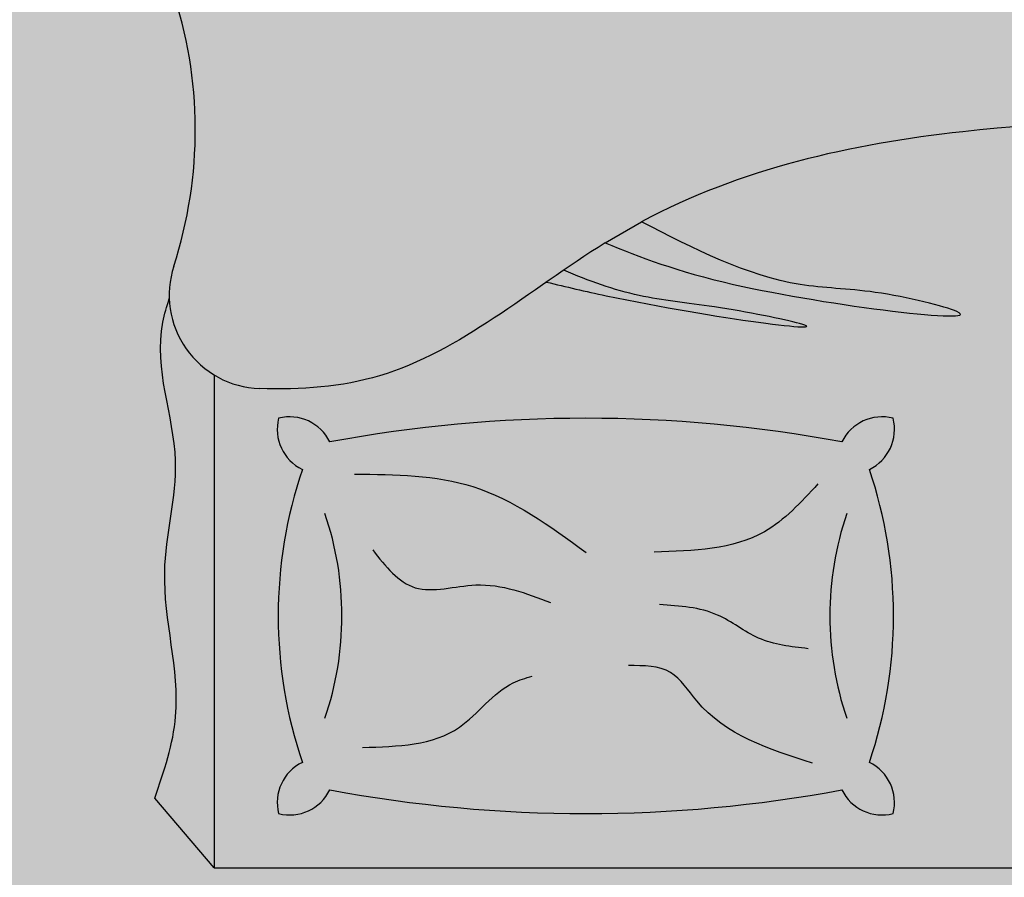
# Model space of a CAD drawing. Units: inches. Extents: x 1704 to 6393, y -157 to 1172.
# Tile 34 of 122: x 2488 to 2529, y 112 to 148. Entities that reach past the tile are written whole.
import ezdxf

# ---------------------------------------------------------------- set-up
doc = ezdxf.new("R2010")
doc.units = ezdxf.units.IN
doc.header["$MEASUREMENT"] = 0
for name, color, linetype, lineweight in [('A-ANNO-DIMS', 7, 'Continuous', 13), ('A-FURN', 8, 'Continuous', 18), ('estofado', 7, 'Continuous', 25)]:
    doc.layers.add(name, color=color, linetype=linetype, lineweight=lineweight)
doc.layers.add('A-FLOR-PATT', color=7, linetype='Continuous', lineweight=13, true_color=0xf2f2f2)
doc.styles.get("Standard").update_dxf_attribs({"font": 'arial.ttf'})
doc.dimstyles.get("Standard").update_dxf_attribs({"dimtxt": 6, "dimasz": 2, "dimexe": 0.18, "dimexo": 0.0625, "dimgap": 0.09, "dimtad": 0, "dimtih": 1, "dimtoh": 1, "dimdec": 1, "dimzin": 0, "dimdsep": 46, "dimlunit": 3, "dimtxsty": 'Standard', "dimblk": 'ARCHTICK', "dimcen": 0.09, "dimadec": 0, "dimazin": 0, "dimtfac": 1, "dimtdec": 1, "dimtofl": 0, "dimtmove": 0, "dimatfit": 3, "dimfxl": 1, "dimtolj": 1, "dimtzin": 0, "dimarcsym": 0})

# ---------------------------------------------------------------- blocks, each defined once
blk = doc.blocks.new('Cama Box Regencia LOLA')
at = {"layer": 'estofado', "ltscale": 0.2}
h = blk.add_hatch(color=256, dxfattribs=at)
h.dxf.hatch_style = 1
h.set_gradient(color1=(240, 232, 219), color2=(213, 190, 154), one_color=1, tint=0.7200000286102295, name='CURVED')
edge = h.paths.add_edge_path()
edge.add_spline(control_points=[(0.343533776195045, -0.8455058148597345), (0.2879313990920309, -0.8167160606696484), (0.2054770794474052, -0.7744470032542381), (0.0954193394759386, -0.7742416952675626), (-0.0885363502328574, -0.7276964167006668), (0.2428192566063672, -0.7672518992321216), (0.345087521536243, -0.8076697826234067), (0.3825206986321063, -0.8228555492498799)], knot_values=[0.0056315103357428, 0.0056315103357428, 0.0056315103357428, 0.0056315103357428, 0.1860138916206105, 0.2660015162584448, 0.3570871810327863, 0.5963901805690979, 0.739731738908988, 0.739731738908988, 0.739731738908988, 0.739731738908988], degree=3, periodic=0)
edge.add_spline(control_points=[(0.3825206986325611, -0.8228555492497662), (0.3974221570828149, -0.8135511441712424), (0.4121061736600496, -0.8037181558521524), (0.4266849906532571, -0.7937075488799225)], knot_values=[1.358237767273279, 1.358237767273279, 1.358237767273279, 1.358237767273279, 1.409915662372559, 1.409915662372559, 1.409915662372559, 1.409915662372559], degree=3, periodic=0)
edge.add_spline(control_points=[(0.4266849905698109, -0.7937075489369932), (0.3998777739682282, -0.7821381809783361), (0.3476761897024971, -0.7634757898491671), (0.2670618099601825, -0.7565375622627358), (0.0835725072796549, -0.7192994417154637), (0.288524529784695, -0.7446405493717521), (0.4247448861246994, -0.7759943071475277), (0.4449816270193879, -0.7810438091316882)], knot_values=[0.1043639306803623, 0.1043639306803623, 0.1043639306803623, 0.1043639306803623, 0.1896363068641149, 0.2696239315019491, 0.3607095962762907, 0.6000125958126024, 0.6446217338078729, 0.6446217338078729, 0.6446217338078729, 0.6446217338078729], degree=3, periodic=0)
edge.add_spline(control_points=[(0.4449816270197289, -0.7810438091316882), (0.5029779388527232, -0.7406836481117695), (0.5966687145296419, -0.6736247633211292), (0.7071737530245628, -0.6656573253703187), (0.7517012483331201, -0.6672238302253392)], knot_values=[1.43159032281798, 1.43159032281798, 1.43159032281798, 1.43159032281798, 1.63814180148235, 1.770695287284994, 1.770695287284994, 1.770695287284994, 1.770695287284994], degree=3, periodic=0)
edge.add_arc((0.7481853615017826, -0.767162003811734), 0.0999999999999888, 58.7920033978138, 87.98512997550938, ccw=False)
edge.add_line((0.8000000000000682, -0.6816328085782289), (0.8000000000000682, -0.154802362840428))
edge.add_line((0.8000000000000682, -0.154802362840428), (-0.7999999999999546, -0.154802362840428))
edge.add_line((-0.7999999999999546, -0.154802362840428), (-0.8000000000000682, -0.7409839258539819))
edge.add_spline(control_points=[(-0.799999999999841, -0.7409839258539251), (-0.7846451382113174, -0.74846387981205), (-0.7568940913494089, -0.7651582159765554), (-0.7559936909002545, -0.8096905380045313), (-0.7049413305308008, -0.8142555457367848), (-0.7013836936888538, -0.8139988647640733)], knot_values=[0.0122267587020837, 0.0122267587020837, 0.0122267587020837, 0.0122267587020837, 0.0594720782072034, 0.1062176618094138, 0.134458043575382, 0.134458043575382, 0.134458043575382, 0.134458043575382], degree=3, periodic=0)
edge.add_spline(control_points=[(-0.7013836936890812, -0.8139988647637892), (-0.6428309483887916, -0.8132695376718857), (-0.532520673001045, -0.8118955240036598), (-0.2390712668254764, -0.6717984706609172), (-0.3892411364554391, -0.7557901092520752), (-0.4591093260188473, -0.8070101468627512), (-0.5571511178645779, -0.795652750469742), (-0.608497950975675, -0.8409486634728295), (-0.6632498050151981, -0.8266781836207997), (-0.6991149398675134, -0.8254126024436914), (-0.719552182989446, -0.8246914287938125)], knot_values=[0, 0, 0, 0, 0.2187005959148062, 0.4120203559900679, 0.4786136596093368, 0.6046444033330721, 0.6969970394608519, 0.7456449795902803, 0.7925683322559657, 0.8547274388453192, 0.8547274388453192, 0.8547274388453192, 0.8547274388453192], degree=3, periodic=0)
edge.add_spline(control_points=[(-0.7195521829781911, -0.824691428792164), (-0.7293124663336812, -0.8248308281530967), (-0.7545977292818407, -0.8216412233076653), (-0.7742556984202338, -0.794819860189591), (-0.7939222919129634, -0.7820064600295497), (-0.799999999999841, -0.7800193173443404)], knot_values=[0.1564883932805935, 0.1564883932805935, 0.1564883932805935, 0.1564883932805935, 0.184397548386913, 0.2313764834161266, 0.2505984550882281, 0.2505984550882281, 0.2505984550882281, 0.2505984550882281], degree=3, periodic=0)
edge.add_line((-0.8000000000000682, -0.7800193173444541), (-0.7999999999999546, -0.8218505664627286))
edge.add_spline(control_points=[(-0.7999999999999546, -0.8218505664625013), (-0.7938082505512511, -0.8290217081292894), (-0.7673857405620766, -0.8512914803976059), (-0.7619109683460011, -0.8661369353891359), (-0.6555700939965164, -0.8510070218793543), (-0.7139793977868294, -0.8637526923380391), (-0.7379026254519659, -0.8623504601624176), (-0.7688129786438367, -0.8813042143888196), (-0.7854260296310259, -0.8561610219318254), (-0.7961930533253962, -0.8566031243811949), (-0.7999999999999546, -0.8573491405791173)], knot_values=[0.0595743221876141, 0.0595743221876141, 0.0595743221876141, 0.0595743221876141, 0.08075289116965, 0.1037414994169835, 0.1697200936249022, 0.1760361327243865, 0.2071371586311508, 0.2404744334261798, 0.2623408547027293, 0.2736604507987723, 0.2736604507987723, 0.2736604507987723, 0.2736604507987723], degree=3, periodic=0)
edge.add_line((-0.7999999999999546, -0.8573491405791173), (-0.8000000000000682, -0.9113562424721521))
edge.add_spline(control_points=[(-0.8000000000000682, -0.9113562424720385), (-0.7937204054647964, -0.9077594990848183), (-0.7710343135782978, -0.8978798065321029), (-0.7213062468074442, -0.9144666877443228), (-0.6268586829058905, -0.862430497409548), (-0.6896594748232019, -0.9045634991654196), (-0.7483442493064559, -0.9189273406958591), (-0.7835301183422417, -0.922920432793262), (-0.7896301351460125, -0.9477657000142585), (-0.7975786973822779, -0.955260590410262), (-0.8000000000001818, -0.9571831923294098)], knot_values=[0.0138560263374175, 0.0138560263374175, 0.0138560263374175, 0.0138560263374175, 0.0348737775836104, 0.0888666909546002, 0.1078792274429341, 0.1267378491223226, 0.1587140219647659, 0.1937574699451985, 0.2174867851300671, 0.2267221218327879, 0.2267221218327879, 0.2267221218327879, 0.2267221218327879], degree=3, periodic=0)
edge.add_line((-0.7999999999999546, -0.957183192329296), (-0.7999999999999546, -1.145824641594742))
edge.add_spline(control_points=[(-0.8000000000002955, -1.145824641594913), (-0.7271039467997298, -1.094596787649038), (-0.4885706936571524, -0.9465888221489535), (-0.0701640902225336, -0.9707493165000187), (0.237911901821235, -0.902164522332157), (0.3435337762145991, -0.845505814843193)], knot_values=[0.1168958193629841, 0.1168958193629841, 0.1168958193629841, 0.1168958193629841, 0.3797203297758731, 0.9577018633805092, 1.31379338443587, 1.31379338443587, 1.31379338443587, 1.31379338443587], degree=3, periodic=0)
h.paths.add_polyline_path([(-0.6766340706021765, -0.6101327540145576, -0.3575266660906883), (-0.7312746368313583, -0.6354535276154252, -0.3575266660894137), (-0.7059538632299791, -0.5808129613865844, -0.1647847126465284), (-0.7059538632300928, -0.2676124402649407, -0.3575266660890756), (-0.7312746368312446, -0.2129718740360431, -0.3575266660908716), (-0.6766340706020629, -0.2382926476369676, -0.0925607043966334), (-0.1295169377724505, -0.2382926476369107, -0.3575266660898965), (-0.0748763715433825, -0.2129718740360431, -0.3575266660894428), (-0.1001971451446479, -0.2676124402649407, -0.1647847126465285), (-0.1001971451445343, -0.5808129613865844, -0.3575266660890756), (-0.0748763715433825, -0.6354535276154821, -0.3575266660898962), (-0.1295169377724505, -0.6101327540146145, -0.0925607043966531)], flags=16)
h.paths.add_polyline_path([(0.0748763715433825, -0.6354535276157094, -0.3575266660910266), (0.1001971451446479, -0.5808129613865844, -0.1647847126465284), (0.1001971451445343, -0.2676124402649407, -0.3575266660890757), (0.0748763715433825, -0.2129718740360431, -0.3575266660898962), (0.1295169377724505, -0.2382926476369107, -0.0925607043966334), (0.6766340706020629, -0.2382926476369676, -0.3575266660908718), (0.7312746368312446, -0.2129718740360431, -0.3575266660894425), (0.7059538632299791, -0.2676124402649407, -0.1647847126465283), (0.7059538632300928, -0.5808129613865844, -0.3575266660890756), (0.7312746368312446, -0.6354535276154821, -0.3575266660908716), (0.6766340706020629, -0.6101327540145576, -0.0925607043966335), (0.1295169377724505, -0.6101327540146145, -0.3575266660906303)], flags=16)
h = blk.add_hatch(color=256, dxfattribs=at)
h.dxf.hatch_style = 1
h.set_gradient(color1=(240, 232, 219), color2=(213, 190, 154), one_color=1, tint=0.7200000286102295)
edge = h.paths.add_edge_path()
edge.add_spline(control_points=[(0.8481164014890509, -0.7634488855285327), (0.8506728373771466, -0.7550468983013161), (0.868679602201837, -0.6953776187201015), (0.8253488717913342, -0.6001498518888299), (0.8674912876568897, -0.4595932758330151), (0.8269013755603964, -0.3369378214810581), (0.8537222782124445, -0.258285373872468), (0.8635971996978923, -0.2293271111754507)], knot_values=[0, 0, 0, 0, 0.0246217641678395, 0.1732110090087366, 0.2929197011275091, 0.4476746021509216, 0.5378548332073604, 0.5378548332073604, 0.5378548332073604, 0.5378548332073604], degree=3, periodic=0)
edge.add_line((0.8635971996978923, -0.229327111175337), (0.8000000000001818, -0.1548023628403712))
edge.add_line((0.8000000000001818, -0.1548023628403712), (0.8000000000000682, -0.681632808574193))
edge.add_arc((0.7481853615026921, -0.7671620038083234), 0.0999999999999888, 2.1279492292164264, 58.79200339844499, ccw=False)
h = blk.add_hatch(color=256, dxfattribs=at)
h.dxf.hatch_style = 1
h.set_gradient(color1=(106, 82, 42), color2=(160, 123, 64), one_color=1, tint=0.4399999976158142, name='CURVED')
h.paths.add_polyline_path([(0.7059538632300928, -0.2676124402650544, 0.3575266660910843), (0.731274636831131, -0.2129718740358157, 0.3575266660898384), (0.6766340706021765, -0.2382926476369107, 0.092560704396653), (0.1295169377724505, -0.2382926476369676, 0.3575266660900799), (0.0748763715433825, -0.2129718740360431, 0.3575266660883129), (0.1001971451444206, -0.2676124402648838, 0.1647847126464969), (0.1001971451445343, -0.5808129613864708, 0.3575266660914516), (0.0748763715433825, -0.6354535276157094, 0.3575266660906303), (0.1295169377724505, -0.6101327540146145, 0.0925607043966335), (0.6766340706020629, -0.6101327540146145, 0.3575266660906881), (0.7312746368312446, -0.6354535276154821, 0.3575266660886796), (0.7059538632300928, -0.5808129613866413, 0.1647847126464968)])
h = blk.add_hatch(color=256, dxfattribs=at)
h.dxf.hatch_style = 1
h.set_gradient(color1=(206, 178, 131), color2=(227, 212, 186), one_color=1, tint=0.8100000023841857, name='CYLINDER')
edge = h.paths.add_edge_path()
edge.add_arc((0.7481853614966667, -0.7671620038115634), 0.0999999999999888, 342.0511336145294, 447.9851299725766)
edge.add_spline(control_points=[(0.7517012483331201, -0.6672238302253392), (0.7071737530245628, -0.6656573253703187), (0.5966687145298692, -0.6736247633211292), (0.5029779388527232, -0.7406836481117125), (0.4449816270195015, -0.7810438091316314)], knot_values=[1.431590322817835, 1.431590322817835, 1.431590322817835, 1.431590322817835, 1.564143808620479, 1.770695287284994, 1.770695287284994, 1.770695287284994, 1.770695287284994], degree=3, periodic=0)
edge.add_spline(control_points=[(0.4449816270195015, -0.7810438091316314), (0.4388957332065502, -0.7852790380018178), (0.4327996148541616, -0.7895089160493285), (0.4266849906533708, -0.7937075488798087)], knot_values=[1.409915662372814, 1.409915662372814, 1.409915662372814, 1.409915662372814, 1.431590322817835, 1.431590322817835, 1.431590322817835, 1.431590322817835], degree=3, periodic=0)
edge.add_spline(control_points=[(0.4266849906533708, -0.7937075488798087), (0.4121061736600496, -0.8037181558521524), (0.3974221570825875, -0.8135511441712991), (0.38252069863222, -0.8228555492498799)], knot_values=[1.358237767273037, 1.358237767273037, 1.358237767273037, 1.358237767273037, 1.409915662372815, 1.409915662372815, 1.409915662372815, 1.409915662372815], degree=3, periodic=0)
edge.add_line((0.3825206986330158, -0.8228555492493114), (0.343533776286904, -0.8455058148063584))
edge.add_spline(control_points=[(0.3435337761924302, -0.8455058148550165), (0.2379119018048641, -0.902164522335795), (-0.0701640902311738, -0.9707493164995071), (-0.4885706936571524, -0.9465888221488967), (-0.7271039467997298, -1.094596787649038), (-0.8000000000000682, -1.145824641594742)], knot_values=[0.1168958193630798, 0.1168958193630798, 0.1168958193630798, 0.1168958193630798, 0.472987340393773, 1.050968873998409, 1.313793384411202, 1.313793384411202, 1.313793384411202, 1.313793384411202], degree=3, periodic=0)
edge.add_spline(control_points=[(-0.8000000000000682, -1.145824641594742), (-0.8038896190357718, -1.14855807951244), (-0.8077744942224853, -1.151305646504738), (-0.8116551946761774, -1.154065647517199)], knot_values=[0.1028719158199011, 0.1028719158199011, 0.1028719158199011, 0.1028719158199011, 0.1168958193630799, 0.1168958193630799, 0.1168958193630799, 0.1168958193630799], degree=3, periodic=0)
edge.add_arc((-0.7536973518524519, -1.235557294053705), 0.1000000000000352, 125.4208969883762, 169.6981795679068)
edge.add_spline(control_points=[(-0.852085287466366, -1.217673946333093), (-0.8521399740518518, -1.217974812833915), (-0.8565649010855622, -1.242328483616745), (-0.8662697220019026, -1.297321141147904), (-0.8487158298532904, -1.34896742172242), (-0.8348745804664758, -1.381844109035796)], knot_values=[0.3128349436863077, 0.3128349436863077, 0.3128349436863077, 0.3128349436863077, 0.3137509534211996, 0.386958004641742, 0.4759027329026081, 0.4759027329026081, 0.4759027329026081, 0.4759027329026081], degree=3, periodic=0)
edge.add_spline(control_points=[(-0.8348745804664758, -1.38184410903591), (-0.8226532004149476, -1.367823298399059), (-0.8056354908857201, -1.352141651537124), (-0.7460155199962628, -1.32170802000337)], knot_values=[0.0062456970656236, 0.0062456970656236, 0.0062456970656236, 0.0062456970656236, 0.0554759259147193, 0.0554759259147193, 0.0554759259147193, 0.0554759259147193], degree=3, periodic=0)
edge.add_spline(control_points=[(-0.7460155200169539, -1.321708019985464), (-0.6188339616464873, -1.25080943574278), (-0.3488365122128698, -1.179158668568902), (0.0338148848931041, -1.279726484458706), (0.3977250465933366, -1.412092721352792), (0.6449024721503065, -1.106270719748692), (0.7873766543807506, -1.256744909425322), (0.8547271521993025, -1.327877176513538)], knot_values=[0.0991852523588446, 0.0991852523588446, 0.0991852523588446, 0.0991852523588446, 0.5236467270390676, 0.9270872950244264, 1.289918234564769, 1.564439021262726, 1.810554634340498, 1.810554634340498, 1.810554634340498, 1.810554634340498], degree=3, periodic=0)
edge.add_arc((0.5509678495186563, -1.223443291813453), 0.3212104454069235, 341.0267878798241, 383.7782184284114)
edge.add_arc((1.292676354991499, -0.9435407756057543), 0.4723459732861395, 162.0511336103901, 198.5657216587827, ccw=False)
h = blk.add_hatch(color=256, dxfattribs=at)
h.dxf.hatch_style = 1
h.set_gradient(color1=(240, 232, 219), color2=(137, 106, 57), one_color=1, tint=0.3799999952316284, name='CURVED')
edge = h.paths.add_edge_path()
edge.add_spline(control_points=[(0.4449816270193879, -0.7810438091316882), (0.4247448861246994, -0.7759943071475277), (0.288524529784695, -0.7446405493717521), (0.0835725072796549, -0.7192994417154637), (0.2670618099601825, -0.7565375622627358), (0.3476761897024971, -0.7634757898491671), (0.3998777739682282, -0.7821381809783361), (0.4266849905698109, -0.7937075489369932)], knot_values=[0.1043639306803623, 0.1043639306803623, 0.1043639306803623, 0.1043639306803623, 0.1489730686756328, 0.3882760682119444, 0.479361732986286, 0.5593493576241202, 0.6446217338078729, 0.6446217338078729, 0.6446217338078729, 0.6446217338078729], degree=3, periodic=0)
edge.add_spline(control_points=[(0.4266849906528023, -0.7937075488800929), (0.4327996148537068, -0.7895089160495559), (0.4388957332062092, -0.7852790380020452), (0.4449816270192742, -0.781043809131802)], knot_values=[1.409915662372559, 1.409915662372559, 1.409915662372559, 1.409915662372559, 1.43159032281798, 1.43159032281798, 1.43159032281798, 1.43159032281798], degree=3, periodic=0)
h = blk.add_hatch(color=256, dxfattribs=at)
h.dxf.hatch_style = 1
h.set_gradient(color1=(240, 232, 219), color2=(137, 106, 57), one_color=1, tint=0.3799999952316284, name='CURVED')
edge = h.paths.add_edge_path()
edge.add_spline(control_points=[(0.3825206986321063, -0.8228555492498799), (0.345087521536243, -0.8076697826234067), (0.2428192566063672, -0.7672518992321216), (-0.0885363502328574, -0.7276964167006668), (0.0954193394759386, -0.7742416952675626), (0.2054770794474052, -0.7744470032542381), (0.2879313990920309, -0.8167160606696484), (0.343533776195045, -0.8455058148597345)], knot_values=[0.0056315103357428, 0.0056315103357428, 0.0056315103357428, 0.0056315103357428, 0.1489730686756328, 0.3882760682119444, 0.479361732986286, 0.5593493576241202, 0.739731738908988, 0.739731738908988, 0.739731738908988, 0.739731738908988], degree=3, periodic=0)
edge.add_line((0.343533776195045, -0.8455058148597913), (0.3825206986321063, -0.8228555492498799))
for p, q in [((0.8000000000000682, -0.154802362840428), (0.8635971996978923, -0.2293271111754507)), ((0.3825206986321063, -0.8228555492498799), (0.343533776195045, -0.8455058148597913))]:
    blk.add_line(p, q, dxfattribs=at)
blk.add_lwpolyline([(0.8000000000000682, -0.6816328085741361), (0.8000000000000682, -0.154802362840428), (-0.7999999999999546, -0.154802362840428), (-0.7999999999999546, -0.7409839258540956)], dxfattribs=at)
for centre, radius, start, end in [((0.120860229745972, -0.2248498560688859), 0.047493175008304, 165.516646303857, 244.209945069049), ((0.0867543535765663, -0.2589557322385758), 0.047493175008304, 25.79005493108792, 104.4833536962803), ((0.4030755041873136, -1.703357436968531), 1.490385562932656, 79.42346065608726, 100.5765393439197), ((0.7193966547980608, -0.2589557322385758), 0.047493175008304, 75.51664630371964, 154.2099450689121), ((0.6852907786285414, -0.2248498560688859), 0.047493175008304, 295.790054930951, 14.48335369614292), ((0.562460708312642, -0.4242127008258194), 0.4880688921049917, 161.2852469077218, 198.7147530922607), ((0.243690300061985, -0.4242127008258194), 0.4880688921049917, 341.2852469077393, 18.71475309227822), ((-0.19631084963396, -0.4242127008257626), 0.3387897965243698, 341.1598423418016, 18.84015765820971), ((1.002461858008359, -0.4242127008257626), 0.3387897965243698, 161.1598423417902, 198.8401576581983), ((0.120860229745972, -0.6235755455826393), 0.047493175008304, 115.790054930951, 194.4833536961429), ((0.6852907786285414, -0.6235755455826393), 0.047493175008304, 345.516646303857, 64.20994506904903), ((0.0867543535765663, -0.5894696694129494), 0.047493175008304, 255.5166463037197, 334.2099450689121), ((0.4030755041873136, 0.8549320353169491), 1.490385562932656, 259.4234606560803, 280.5765393439127), ((0.7193966547980608, -0.5894696694129494), 0.047493175008304, 205.7900549310879, 284.4833536962804), ((0.7481853615029195, -0.7671620038083234), 0.1, 342.0511336116027, 87.98512997616182), ((1.292676354991613, -0.9435407756055268), 0.4723459732861117, 162.0511336104213, 198.5657216589983)]:
    blk.add_arc(centre, radius, start, end, dxfattribs=at)
for points, knots in [([(0.8635971996978923, -0.2293271111754507), (0.8537222782124445, -0.258285373872468), (0.8269013755603964, -0.3369378214810581), (0.8674912876568897, -0.4595932758330151), (0.8253488717913342, -0.6001498518888299), (0.868679602201837, -0.6953776187201015), (0.8506728373771466, -0.7550468983013161), (0.8481164014890509, -0.7634488855285327)], [0, 0, 0, 0, 0.0901802310564388, 0.2449351320798513, 0.3646438241986237, 0.5132330690395209, 0.5378548332073604, 0.5378548332073604, 0.5378548332073604, 0.5378548332073604]), ([(0.1609929429250769, -0.2668120520876869), (0.207361296664481, -0.2816189425177519), (0.2673465842344797, -0.3007741531050562), (0.3100088172549912, -0.3711986237053177), (0.3410959220547441, -0.371113456673647), (0.3573768361287648, -0.371068853062809)], [0, 0, 0, 0, 0.1404794637529129, 0.1817338842404631, 0.2270973195475621, 0.2270973195475621, 0.2270973195475621, 0.2270973195475621]), ([(0.641547568925148, -0.2836087781224137), (0.6039704843628328, -0.2846768301159754), (0.539944686002343, -0.2864966328594507), (0.4983244357833337, -0.3487001107148991), (0.4673537235191868, -0.3577134183149331), (0.460449429265168, -0.3597227530484019)], [0, 0, 0, 0, 0.1057518620258909, 0.1801855432155129, 0.2015394496060149, 0.2015394496060149, 0.2015394496060149, 0.2015394496060149]), ([(0.1657269282603693, -0.3891622340328808), (0.1839821155447316, -0.3912290170364152), (0.2191851220416109, -0.3952145677934529), (0.2641538569791404, -0.4324302667024541), (0.3028411853428648, -0.4348886966416372), (0.3243911361614664, -0.4362581125853354)], [0, 0, 0, 0, 0.0540396012867365, 0.1042090889319622, 0.1672963371706364, 0.1672963371706364, 0.1672963371706364, 0.1672963371706364]), ([(0.630774277431101, -0.4946666993113809), (0.6169895699779718, -0.4772535648042688), (0.5885015945383536, -0.441266950663047), (0.5131074616321869, -0.4662255111125919), (0.4667910825139399, -0.4484404284426592), (0.4408934738504513, -0.4384959742387196)], [0, 0, 0, 0, 0.0606588350328579, 0.1253597443752535, 0.2074214353097695, 0.2074214353097695, 0.2074214353097695, 0.2074214353097695]), ([(0.1552772464440295, -0.5652394970176715), (0.1730924483668451, -0.5457941389807961), (0.2188221854511549, -0.4958799637506091), (0.2880058022633399, -0.4937226941133118), (0.3302371516485891, -0.4924058446629829)], [0, 0, 0, 0, 0.0765478869158952, 0.1964903209174588, 0.1964903209174588, 0.1964903209174588, 0.1964903209174588]), ([(0.6501439432536245, -0.5758072434303472), (0.6067249420939599, -0.5753127958675333), (0.5155219215609228, -0.5742741927209986), (0.4416129136043037, -0.5203678897559305), (0.402889750189047, -0.4921247481343585)], [0, 0, 0, 0, 0.1270530108164939, 0.2668789710677518, 0.2668789710677518, 0.2668789710677518, 0.2668789710677518]), ([(0.38252069863222, -0.8228555492498799), (0.4632317710900225, -0.7724599107979202), (0.5727651217678158, -0.6753482176968646), (0.7071737530245628, -0.6656573253703187), (0.7517012483331201, -0.6672238302253392)], [1.358237767273037, 1.358237767273037, 1.358237767273037, 1.358237767273037, 1.63814180148235, 1.770695287284994, 1.770695287284994, 1.770695287284994, 1.770695287284994]), ([(0.4449816270193879, -0.7810438091316882), (0.4247448861246994, -0.7759943071475277), (0.288524529784695, -0.7446405493717521), (0.0835725072796549, -0.7192994417154637), (0.2670618099601825, -0.7565375622627358), (0.3476761897024971, -0.7634757898491671), (0.3998777739682282, -0.7821381809783361), (0.4266849905698109, -0.7937075489369932)], [0.1043639306803623, 0.1043639306803623, 0.1043639306803623, 0.1043639306803623, 0.1489730686756328, 0.3882760682119444, 0.479361732986286, 0.5593493576241202, 0.6446217338078729, 0.6446217338078729, 0.6446217338078729, 0.6446217338078729]), ([(0.3825206986321063, -0.8228555492498799), (0.345087521536243, -0.8076697826234067), (0.2428192566063672, -0.7672518992321216), (-0.0885363502328574, -0.7276964167006668), (0.0954193394759386, -0.7742416952675626), (0.2054770794474052, -0.7744470032542381), (0.2879313990920309, -0.8167160606696484), (0.343533776195045, -0.8455058148597345)], [0.0056315103357428, 0.0056315103357428, 0.0056315103357428, 0.0056315103357428, 0.1489730686756328, 0.3882760682119444, 0.479361732986286, 0.5593493576241202, 0.739731738908988, 0.739731738908988, 0.739731738908988, 0.739731738908988]), ([(-0.8116551946761774, -1.154065647517199), (-0.7350455857787211, -1.099579968801037), (-0.493473113061782, -0.9463057365681493), (-0.0701640902311738, -0.9707493164995071), (0.2379119018048641, -0.902164522335795), (0.3435337761924302, -0.8455058148550165)], [0.1028719158199011, 0.1028719158199011, 0.1028719158199011, 0.1028719158199011, 0.3797203297758731, 0.9577018633805092, 1.313793384411202, 1.313793384411202, 1.313793384411202, 1.313793384411202])]:
    blk.add_open_spline(points, degree=3, knots=knots, dxfattribs=at)
blk = doc.blocks.new('_ArchTick')
at = {"color": 0, "linetype": 'ByBlock', "const_width": 0.15}
blk.add_lwpolyline([(-0.5, -0.5), (0.5, 0.5)], dxfattribs=at)
blk = doc.blocks.new('*D93')
at = {"layer": 'A-ANNO-DIMS', "color": 0, "lineweight": -2, "transparency": 16777216}
for p, q in [((2605.286074000001, 895.2129740000005), (1829.697551000002, 895.2129740000003)), ((1829.877551000002, 895.2129740000003), (1829.877551000002, 495.8664119263302)), ((1829.877551000002, 90.2129739999999), (1829.877551000002, 489.5595360736699)), ((2605.286074000001, 90.21297400000003), (1829.697551000002, 90.2129739999999))]:
    blk.add_line(p, q, dxfattribs=at)
at = {"layer": 'Defpoints', "color": 0, "lineweight": -3, "transparency": 16777216}
for p in [(2605.348574000001, 895.2129740000005), (1829.877551000002, 90.2129739999999), (2605.348574000001, 90.21297400000003)]:
    blk.add_point(p, dxfattribs=at)
at = {"layer": 'A-ANNO-DIMS', "color": 0, "lineweight": -2, "transparency": 16777216, "xscale": 2, "yscale": 2, "zscale": 2}
for p, rotation in [((1829.877551000002, 895.2129740000003), 90), ((1829.877551000002, 90.2129739999999), 270)]:
    blk.add_blockref('_ArchTick', p, dxfattribs=dict(at, rotation=rotation))
at = {"layer": 'A-ANNO-DIMS', "color": 0, "transparency": 16777216, "insert": (1829.877551000001, 492.7129739999994), "char_height": 6, "attachment_point": 5}
blk.add_mtext('\\A1;805', dxfattribs=at)
blk = doc.blocks.new('*D105')
at = {"layer": 'A-ANNO-DIMS', "color": 0, "lineweight": -2, "transparency": 16777216}
for p, q in [((2451.737975, 615.150474), (2451.737975, -64.9670259999999)), ((2547.348574, 615.150474), (2547.348574, -64.9670259999999)), ((2451.737975, -64.787026), (2489.908936164393, -64.787026)), ((2547.348574, -64.787026), (2509.177612835607, -64.787026))]:
    blk.add_line(p, q, dxfattribs=at)
at = {"layer": 'Defpoints', "color": 0, "lineweight": -3, "transparency": 16777216}
for p in [(2451.737975, 615.212974), (2547.348574, 615.212974), (2547.348574, -64.787026)]:
    blk.add_point(p, dxfattribs=at)
at = {"layer": 'A-ANNO-DIMS', "color": 0, "lineweight": -2, "transparency": 16777216, "xscale": 2, "yscale": 2, "zscale": 2, "rotation": 180}
blk.add_blockref('_ArchTick', (2451.737975, -64.787026), dxfattribs=at)
at = {"layer": 'A-ANNO-DIMS', "color": 0, "lineweight": -2, "transparency": 16777216, "xscale": 2, "yscale": 2, "zscale": 2}
blk.add_blockref('_ArchTick', (2547.348574, -64.787026), dxfattribs=at)
at = {"layer": 'A-ANNO-DIMS', "color": 0, "transparency": 16777216, "insert": (2499.5432745, -64.787026), "char_height": 6, "attachment_point": 5}
blk.add_mtext('\\A1;95.61', dxfattribs=at)

msp = doc.modelspace()

# ---------------------------------------------------------------- hatches: boundary and pattern name
at = {"layer": 'A-FLOR-PATT', "transparency": 33554528}
h = msp.add_hatch(color=256, dxfattribs=at)
h.dxf.hatch_style = 1
h.paths.add_polyline_path([(2325.348574056059, 863.2129735309796), (2325.348574056059, 887.2129735309796), (2263.348574056059, 887.2129735309796), (2167.348574056059, 887.2129735309794), (2081.348574056061, 887.2129735309792), (2081.348574056061, 719.2129735309785), (2277.348574056059, 719.2129735309787), (2277.348574056059, 711.2129735309788), (2277.348574056059, 372.212973530979), (2349.348574056059, 372.212973530979), (2381.348574056059, 372.2129735309789), (2381.348574056059, 364.2129735309789), (2353.348574056059, 364.2129735309789), (2353.348574056059, 270.2129735309788), (2381.348574056059, 270.2129735309788), (2381.348574056059, 266.2129735309788), (2357.348574056059, 266.2129735309788), (2357.348574056059, 98.21297353097884), (2381.348574056059, 98.21297353097897), (2385.181056550604, 98.21297353097884), (2386.482186711948, 98.21297353097884), (2424.21496140017, 98.21297353097884), (2425.516091561514, 98.21297353097884), (2429.348574056059, 98.21297353097897), (2597.348574056059, 98.21297353097884), (2597.348574056059, 146.2129735309788), (2597.348574056059, 218.2129735309788), (2597.348574056059, 266.2129735309788), (2423.348574056059, 266.2129735309788), (2423.348574056059, 270.2129735309788), (2473.348574056059, 270.2129735309788), (2473.348574056059, 294.2129735309789), (2477.348574056059, 294.2129735309789), (2477.348574056059, 270.2129735309788), (2547.348574056059, 270.2129735309788), (2547.348574056059, 364.2129735309788), (2477.348574056059, 364.2129735309788), (2477.348574056059, 318.2129735309788), (2473.348574056059, 318.2129735309787), (2473.348574056059, 364.2129735309789), (2423.348574056059, 364.2129735309788), (2423.348574056059, 372.2129735309788), (2469.348574056059, 372.2129735309788), (2469.348574056059, 459.2129735309789), (2469.348574056059, 538.2129735309788), (2350.348574056059, 538.2129735309788), (2350.348574056059, 565.7129735309788), (2358.348574056059, 565.7129735309788), (2358.348574056059, 545.2129735309788), (2420.348574056059, 545.2129735309788), (2420.348574056059, 610.2129735309788), (2358.348574056059, 610.2129735309788), (2358.348574056059, 589.7129735309788), (2350.348574056059, 589.7129735309788), (2350.348574056059, 615.2129735309788), (2425.348574056059, 615.2129735309788), (2425.348574056059, 607.2129735309788), (2425.348574056059, 546.2129735309788), (2469.348574056059, 546.2129735309788), (2514.34857405606, 546.212973530979), (2514.34857405606, 607.2129735309788), (2449.348574056059, 607.2129735309788), (2449.348574056059, 615.2129735309788), (2451.737974987759, 615.2129735309788), (2451.737974987759, 659.2129735309788), (2427.737974987759, 659.2129735309788), (2427.737974987759, 665.2129735309788), (2367.737974987758, 665.2129735309788), (2367.737974987758, 667.2129735309788), (2367.737974987758, 711.2129735309788), (2325.348574056059, 711.2129735309788), (2325.348574056059, 719.2129735309785), (2325.348574056059, 755.2129735309787), (2325.348574056059, 763.2129735309788)])
h.paths.add_polyline_path([(2233.85817000392, 822.532660166629, -0.1872470486944155), (2233.85817000392, 809.1396667958562), (2231.697030374885, 808.8044951349628, 0.0848927708004382), (2233.130501812631, 814.4858417746204), (2230.423974436808, 814.4858417746204, -0.1042581087707907), (2228.553363812687, 808.3129425443484), (2217.750790159711, 807.1555239386723, -0.2222222222222219), (2217.750790159711, 824.5168030238124), (2228.553363812687, 823.3593844181363, -0.1042581087707933), (2230.423974436808, 817.1864851878643), (2233.130501812631, 817.1864851878643, 0.08489277080044), (2231.697030374885, 822.8678318275219)], flags=16)
h.paths.add_polyline_path([(2213.621360876743, 833.1974425663823), (2213.621360876743, 798.4748843961024), (2156.047684459484, 798.4748843961034), (2156.047684459485, 833.1974425663813)], flags=16)
h.paths.add_polyline_path([(2203.931929661768, 848.0987249710489), (2205.089348267444, 837.2961513180724, -0.2222222222222264), (2187.728069182304, 837.2961513180724), (2188.88548778798, 848.0987249710485, -0.104258108770792), (2195.058387018252, 849.9693355951691), (2195.058387018252, 852.6758629709927, 0.084892770800438), (2189.377040378595, 851.2423915332469), (2189.712212039488, 853.4035311622828, -0.1872470486944166), (2203.105205410261, 853.4035311622828), (2203.440377071154, 851.2423915332469, 0.084892770800438), (2197.759030431496, 852.6758629709927), (2197.759030431496, 849.9693355951691, -0.1042581087707896)], flags=16)
h.paths.add_polyline_path([(2181.940976153924, 837.2961513180726, -0.2222222222222323), (2164.579697068783, 837.2961513180724), (2165.73711567446, 848.0987249710487, -0.1042581087707905), (2171.910014904732, 849.9693355951691), (2171.910014904732, 852.6758629709927, 0.0848927708004445), (2166.228668265074, 851.2423915332469), (2166.563839925967, 853.403531162283, -0.1872470486944096), (2179.95683329674, 853.4035311622828), (2180.292004957633, 851.2423915332465, 0.0848927708004458), (2174.610658317976, 852.6758629709927), (2174.610658317976, 849.9693355951691, -0.104258108770801), (2180.783557548248, 848.0987249710482)], flags=16)
h.paths.add_polyline_path([(2205.089348267444, 794.376175644412), (2203.931929661768, 783.5736019914364, -0.1042581087707934), (2197.759030431496, 781.7029913673155), (2197.759030431496, 778.9964639914921, 0.084892770800439), (2203.440377071154, 780.4299354292382), (2203.105205410261, 778.2687958002022, -0.1872470486944172), (2189.712212039488, 778.2687958002018), (2189.377040378595, 780.4299354292377, 0.0848927708004369), (2195.058387018252, 778.9964639914919), (2195.058387018252, 781.7029913673153, -0.1042581087707904), (2188.88548778798, 783.5736019914358), (2187.728069182304, 794.3761756444126, -0.2222222222222231)], flags=16)
h.paths.add_polyline_path([(2181.940976153924, 794.376175644412), (2180.783557548248, 783.5736019914364, -0.1042581087708008), (2174.610658317976, 781.7029913673153), (2174.610658317976, 778.9964639914921, 0.0848927708004458), (2180.292004957633, 780.4299354292382), (2179.95683329674, 778.268795800202, -0.1872470486944096), (2166.563839925967, 778.2687958002018), (2166.228668265074, 780.4299354292378, 0.0848927708004446), (2171.910014904732, 778.9964639914919), (2171.910014904732, 781.7029913673153, -0.1042581087707904), (2165.73711567446, 783.5736019914358), (2164.579697068783, 794.3761756444123, -0.2222222222222294)], flags=16)
h.paths.add_polyline_path([(2151.918255176517, 807.1555239386723), (2141.115681523541, 808.3129425443484, -0.1042581087707911), (2139.24507089942, 814.4858417746204), (2136.538543523597, 814.4858417746204, 0.08489277080044), (2137.972014961343, 808.8044951349626), (2135.810875332307, 809.1396667958562, -0.1872470486944109), (2135.810875332307, 822.5326601666285), (2137.972014961343, 822.8678318275221, 0.0848927708004416), (2136.538543523597, 817.1864851878643), (2139.24507089942, 817.1864851878643, -0.104258108770793), (2141.115681523541, 823.3593844181363), (2151.918255176517, 824.5168030238124, -0.2222222222222205)], flags=16)
h.paths.add_polyline_path([(2357.868011454448, 363.4102250290031), (2358.813881560335, 363.4102250290031, 0.7537604849588476)], flags=16)
h.paths.add_polyline_path([(2372.241054283868, 363.1167008961685), (2372.248110816919, 363.1167008961685), (2372.248110816919, 363.3425764997267), (2371.30224071103, 363.3425764997267), (2371.30224071103, 363.1392706554335, -1.360391292333951)], flags=16)
h.paths.add_polyline_path([(2371.309297244092, 272.7157694655011), (2371.30224071103, 272.7157694655011), (2371.30224071103, 272.4898938619428), (2372.248110816919, 272.4898938619428), (2372.248110816919, 272.6931997062759, -1.360391292393621)], flags=16)
h.paths.add_polyline_path([(2357.875067987504, 272.7157694655011), (2357.868011454452, 272.7157694655011), (2357.868011454452, 272.4898938619428), (2358.813881560341, 272.4898938619428), (2358.813881560341, 272.6931997062361, -1.360391292333948)], flags=16)
h.paths.add_polyline_path([(2353.768696905258, 363.0736921025416), (2376.347425366111, 363.0736921025416), (2376.347425366111, 272.7587782591281), (2353.768696905258, 272.7587782591281)], flags=16)
h.paths.add_polyline_path([(2354.772195947961, 362.0701930598379), (2375.343926323407, 362.0701930598379), (2375.343926323407, 273.7622773018316), (2354.772195947961, 273.7622773018318)], flags=0)
h.paths.add_polyline_path([(2357.868011454452, 363.3425764997267), (2358.813881560341, 363.3425764997266), (2358.813881560341, 363.1167008961684), (2357.868011454452, 363.1167008961684)], flags=16)
h.paths.add_polyline_path([(2359.287941640134, 359.1843485433627), (2359.287941640134, 360.0631949744305), (2370.828180631237, 360.0631949744362), (2370.828180631237, 359.1843485433769), (2374.332057422314, 359.1843485433812), (2374.332057422312, 358.4635369582513), (2372.835178716611, 358.4635369582524), (2372.835178716611, 357.5410357047662), (2374.332057422314, 357.5410357047678), (2374.332057422312, 356.8202241196381), (2372.835178716611, 356.820224119639), (2372.835178716611, 355.897722866153), (2374.332057422314, 355.8977228661546), (2374.332057422312, 355.1769112810248), (2372.835178716611, 355.1769112810259), (2372.835178716611, 354.2544100275397), (2374.332057422334, 354.2544100275415), (2374.332057422331, 353.5335984424117), (2372.835178716631, 353.5335984424126), (2372.835178716631, 352.6110971889265), (2374.332057422334, 352.6110971889282), (2374.332057422331, 351.8902856037984), (2372.835178716631, 351.8902856037993), (2372.835178716631, 350.9677843503132), (2374.332057422334, 350.967784350315), (2374.332057422331, 350.2469727651852), (2372.835178716631, 350.2469727651861), (2372.835178716631, 349.3244715117), (2374.332057422334, 349.3244715117017), (2374.332057422331, 348.603659926572), (2372.835178716631, 348.6036599265729), (2372.835178716631, 347.6811586730868), (2374.332057422334, 347.6811586730886), (2374.332057422331, 346.9603470879587), (2372.835178716631, 346.9603470879598), (2372.835178716631, 346.0378458344735), (2374.332057422334, 346.0378458344753), (2374.332057422331, 345.3170342493456), (2372.835178716631, 345.3170342493465), (2372.835178716631, 344.3945329958605), (2374.332057422334, 344.3945329958621), (2374.332057422331, 343.6737214107324), (2372.835178716631, 343.6737214107334), (2372.835178716631, 342.751220157247), (2374.332057422334, 342.7512201572489), (2374.332057422331, 342.0304085721191), (2372.835178716631, 342.03040857212), (2372.835178716631, 341.1079073186338), (2374.332057422334, 341.1079073186356), (2374.332057422331, 340.3870957335057), (2372.835178716631, 340.3870957335066), (2372.835178716631, 339.4645944800207), (2374.332057422334, 339.4645944800223), (2374.332057422331, 338.7437828948924), (2372.835178716648, 338.7437828948933), (2372.835178716648, 337.8212816414076), (2374.332057422334, 337.8212816414093), (2374.332057422331, 337.1004700562794), (2372.835178716648, 337.1004700562803), (2372.835178716648, 336.1779688027942), (2374.332057422334, 336.1779688027961), (2374.332057422331, 335.4571572176662), (2372.835178716648, 335.4571572176673), (2372.835178716648, 334.5346559641809), (2374.332057422334, 334.5346559641828), (2374.332057422331, 333.8138443790529), (2372.835178716648, 333.8138443790539), (2372.835178716648, 332.8913431255679), (2374.332057422334, 332.8913431255696), (2374.332057422331, 332.1705315404397), (2372.835178716648, 332.1705315404406), (2372.835178716648, 331.2480302869545), (2374.332057422334, 331.2480302869563), (2374.332057422331, 330.5272187018265), (2372.835178716648, 330.5272187018273), (2372.835178716648, 329.6047174483413), (2374.332057422334, 329.6047174483431), (2374.332057422331, 328.8839058632133), (2372.835178716648, 328.8839058632143), (2372.835178716648, 327.9614046097282), (2374.332057422334, 327.9614046097298), (2374.332057422331, 327.2405930246), (2372.835178716648, 327.2405930246009), (2372.835178716648, 326.3180917711149), (2374.332057422334, 326.3180917711167), (2374.332057422331, 325.5972801859869), (2372.835178716648, 325.5972801859877), (2372.835178716648, 324.6747789325016), (2374.332057422334, 324.6747789325034), (2374.332057422331, 323.9539673473736), (2372.835178716648, 323.9539673473746), (2372.835178716648, 323.0314660938884), (2374.332057422334, 323.0314660938901), (2374.332057422331, 322.3106545087603), (2372.835178716648, 322.3106545087613), (2372.835178716648, 321.3881532552753), (2374.332057422334, 321.388153255277), (2374.332057422331, 320.6673416701471), (2372.835178716648, 320.6673416701481), (2372.835178716648, 319.7448404166621), (2374.332057422334, 319.7448404166638), (2374.332057422331, 319.0240288315339), (2372.835178716648, 319.0240288315348), (2372.835178716648, 318.1015275780487), (2374.332057422334, 318.1015275780504), (2374.332057422331, 317.3807159929205), (2372.835178716648, 317.3807159929214), (2372.835178716648, 316.4582147394357), (2374.332057422334, 316.4582147394373), (2374.332057422331, 315.7374031543073), (2372.835178716648, 315.7374031543084), (2372.835178716648, 314.8149019008223), (2374.332057422334, 314.8149019008241), (2374.332057422331, 314.0940903156943), (2372.835178716648, 314.0940903156952), (2372.835178716648, 313.171589062209), (2374.332057422334, 313.1715890622108), (2374.332057422331, 312.450777477081), (2372.835178716648, 312.4507774770819), (2372.835178716648, 311.5282762235959), (2374.332057422334, 311.5282762235977), (2374.332057422331, 310.8074646384678), (2372.835178716648, 310.8074646384687), (2372.835178716648, 309.8849633849827), (2374.332057422334, 309.8849633849844), (2374.332057422331, 309.1641517998546), (2372.835178716648, 309.1641517998555), (2372.835178716648, 308.2416505463693), (2374.332057422334, 308.2416505463712), (2374.332057422331, 307.5208389612412), (2372.835178716648, 307.5208389612421), (2372.835178716648, 306.5983377077562), (2374.332057422334, 306.598337707758), (2374.332057422331, 305.8775261226281), (2372.835178716648, 305.8775261226289), (2372.835178716648, 304.955024869143), (2374.332057422334, 304.9550248691447), (2374.332057422331, 304.2342132840149), (2372.835178716648, 304.2342132840158), (2372.835178716648, 303.3117120305298), (2374.332057422334, 303.3117120305316), (2374.332057422331, 302.5909004454018), (2372.835178716648, 302.5909004454027), (2372.835178716648, 301.6683991919165), (2374.332057422334, 301.6683991919183), (2374.332057422331, 300.9475876067885), (2372.835178716648, 300.9475876067894), (2372.835178716648, 300.0250863533033), (2374.332057422334, 300.025086353305), (2374.332057422331, 299.3042747681752), (2372.835178716648, 299.3042747681761), (2372.835178716648, 298.3817735146902), (2374.332057422334, 298.3817735146919), (2374.332057422331, 297.6609619295621), (2372.835178716648, 297.6609619295629), (2372.835178716648, 296.7384606760769), (2374.332057422334, 296.7384606760786), (2374.332057422331, 296.0176490909488), (2372.835178716648, 296.0176490909498), (2372.835178716648, 295.0951478374636), (2374.332057422334, 295.0951478374653), (2374.332057422331, 294.3743362523355), (2372.835178716648, 294.3743362523364), (2372.835178716648, 293.4518349988504), (2374.332057422334, 293.4518349988522), (2374.332057422331, 292.7310234137224), (2372.835178716648, 292.7310234137233), (2372.835178716648, 291.8085221602371), (2374.332057422334, 291.8085221602389), (2374.332057422331, 291.0877105751091), (2372.835178716648, 291.08771057511), (2372.835178716648, 290.165209321624), (2374.332057422334, 290.1652093216256), (2374.332057422331, 289.4443977364957), (2372.835178716648, 289.4443977364966), (2372.835178716648, 288.5218964830108), (2374.332057422334, 288.5218964830125), (2374.332057422331, 287.8010848978827), (2372.835178716648, 287.8010848978836), (2372.835178716648, 286.8785836443975), (2374.332057422334, 286.8785836443993), (2374.332057422331, 286.1577720592695), (2372.835178716648, 286.1577720592703), (2372.835178716648, 285.2352708057842), (2374.332057422334, 285.2352708057861), (2374.332057422331, 284.5144592206562), (2372.835178716648, 284.514459220657), (2372.835178716648, 283.5919579671712), (2374.332057422334, 283.5919579671728), (2374.332057422331, 282.871146382043), (2372.835178716648, 282.8711463820439), (2372.835178716648, 281.9486451285579), (2374.332057422334, 281.9486451285596), (2374.332057422331, 281.2278335434298), (2372.835178716648, 281.2278335434307), (2372.835178716648, 280.3053322899446), (2374.332057422334, 280.3053322899464), (2374.332057422331, 279.5845207048164), (2372.835178716648, 279.5845207048174), (2372.835178716648, 278.6620194513314), (2374.332057422334, 278.6620194513331), (2374.332057422331, 277.9412078662033), (2372.835178716648, 277.9412078662043), (2372.835178716648, 277.0187066127184), (2374.332057422334, 277.0187066127201), (2374.332057422331, 276.29789502759), (2370.828180631244, 276.2978950275922), (2370.828180631244, 275.7692753872335), (2359.287941640128, 275.7692753872392), (2359.287941640128, 276.2978950275993), (2355.784064849037, 276.2978950276015), (2355.784064849037, 277.0187066126971), (2357.280943554723, 277.0187066126989), (2357.280943554723, 277.9412078662137), (2355.784064849037, 277.9412078662145), (2355.784064849037, 278.6620194513103), (2357.280943554723, 278.6620194513122), (2357.280943554723, 279.5845207048271), (2355.784064849037, 279.584520704828), (2355.784064849037, 280.3053322899236), (2357.280943554723, 280.3053322899253), (2357.280943554723, 281.2278335434403), (2355.784064849037, 281.2278335434412), (2355.784064849037, 281.9486451285369), (2357.280943554723, 281.9486451285387), (2357.280943554723, 282.8711463820535), (2355.784064849037, 282.8711463820543), (2355.784064849037, 283.5919579671501), (2357.280943554723, 283.591957967152), (2357.280943554723, 284.5144592206668), (2355.784064849037, 284.5144592206676), (2355.784064849037, 285.2352708057632), (2357.280943554723, 285.2352708057651), (2357.280943554723, 286.1577720592801), (2355.784064849037, 286.1577720592809), (2355.784064849037, 286.8785836443766), (2357.280943554723, 286.8785836443784), (2357.280943554723, 287.8010848978931), (2355.784064849037, 287.8010848978941), (2355.784064849037, 288.5218964829895), (2357.280943554723, 288.5218964829913), (2357.280943554723, 289.4443977365064), (2355.784064849037, 289.4443977365072), (2355.784064849037, 290.1652093216029), (2357.280943554723, 290.1652093216047), (2357.280943554723, 291.0877105751197), (2355.784064849037, 291.0877105751206), (2355.784064849037, 291.8085221602161), (2357.280943554723, 291.8085221602179), (2357.280943554723, 292.7310234137328), (2355.784064849037, 292.7310234137337), (2355.784064849037, 293.4518349988293), (2357.280943554723, 293.451834998831), (2357.280943554723, 294.3743362523461), (2355.784064849037, 294.3743362523469), (2355.784064849037, 295.0951478374426), (2357.280943554723, 295.0951478374445), (2357.280943554723, 296.0176490909594), (2355.784064849037, 296.0176490909601), (2355.784064849037, 296.7384606760557), (2357.280943554723, 296.7384606760575), (2357.280943554723, 297.6609619295724), (2355.784064849037, 297.6609619295734), (2355.784064849037, 298.3817735146691), (2357.280943554723, 298.3817735146709), (2357.280943554723, 299.3042747681858), (2355.784064849037, 299.3042747681866), (2355.784064849037, 300.0250863532823), (2357.280943554723, 300.0250863532841), (2357.280943554723, 300.9475876067989), (2355.784064849037, 300.9475876067997), (2355.784064849037, 301.6683991918954), (2357.280943554723, 301.6683991918973), (2357.280943554723, 302.5909004454123), (2355.784064849037, 302.5909004454133), (2355.784064849037, 303.3117120305088), (2357.280943554723, 303.3117120305105), (2357.280943554723, 304.2342132840254), (2355.784064849037, 304.2342132840262), (2355.784064849037, 304.9550248691219), (2357.280943554723, 304.9550248691238), (2357.280943554723, 305.8775261226386), (2355.784064849037, 305.8775261226394), (2355.784064849037, 306.5983377077352), (2357.280943554723, 306.5983377077369), (2357.280943554723, 307.5208389612518), (2355.784064849037, 307.5208389612528), (2355.784064849037, 308.2416505463484), (2357.280943554723, 308.2416505463501), (2357.280943554723, 309.1641517998652), (2355.784064849037, 309.1641517998661), (2355.784064849037, 309.8849633849617), (2357.280943554723, 309.8849633849634), (2357.280943554723, 310.8074646384782), (2355.784064849037, 310.8074646384791), (2355.784064849037, 311.5282762235748), (2357.280943554723, 311.5282762235767), (2357.280943554723, 312.4507774770916), (2355.784064849037, 312.4507774770925), (2355.784064849037, 313.171589062188), (2357.280943554723, 313.1715890621898), (2357.280943554723, 314.0940903157049), (2355.784064849037, 314.0940903157058), (2355.784064849037, 314.8149019008013), (2357.280943554723, 314.8149019008032), (2357.280943554723, 315.7374031543179), (2355.784064849037, 315.7374031543187), (2355.784064849037, 316.4582147394146), (2357.280943554723, 316.4582147394165), (2357.280943554723, 317.3807159929311), (2355.784064849037, 317.3807159929321), (2355.784064849037, 318.1015275780277), (2357.280943554723, 318.1015275780295), (2357.280943554723, 319.0240288315445), (2355.784064849037, 319.0240288315454), (2355.784064849037, 319.744840416641), (2357.280943554723, 319.7448404166428), (2357.280943554723, 320.6673416701576), (2355.784064849037, 320.6673416701585), (2355.784064849037, 321.3881532552541), (2357.280943554723, 321.388153255256), (2357.280943554723, 322.3106545087708), (2355.784064849037, 322.3106545087718), (2355.784064849037, 323.0314660938674), (2357.280943554723, 323.0314660938692), (2357.280943554723, 323.9539673473843), (2355.784064849037, 323.9539673473851), (2355.784064849037, 324.6747789324806), (2357.280943554723, 324.6747789324824), (2357.280943554723, 325.5972801859974), (2355.784064849037, 325.5972801859983), (2355.784064849037, 326.3180917710939), (2357.280943554723, 326.3180917710958), (2357.280943554723, 327.2405930246105), (2355.784064849037, 327.2405930246113), (2355.784064849037, 327.9614046097071), (2357.280943554723, 327.961404609709), (2357.280943554723, 328.8839058632238), (2355.784064849037, 328.8839058632245), (2355.784064849037, 329.6047174483202), (2357.280943554723, 329.604717448322), (2357.280943554723, 330.527218701837), (2355.784064849037, 330.5272187018379), (2355.784064849037, 331.2480302869335), (2357.280943554723, 331.2480302869353), (2357.280943554723, 332.1705315404502), (2355.784064849037, 332.170531540451), (2355.784064849037, 332.8913431255468), (2357.280943554723, 332.8913431255486), (2357.280943554723, 333.8138443790634), (2355.784064849037, 333.8138443790642), (2355.784064849037, 334.5346559641599), (2357.280943554723, 334.5346559641618), (2357.280943554723, 335.4571572176767), (2355.784064849037, 335.4571572176776), (2355.784064849037, 336.1779688027732), (2357.280943554723, 336.177968802775), (2357.280943554723, 337.1004700562898), (2355.784064849037, 337.1004700562908), (2355.784064849037, 337.8212816413864), (2357.280943554723, 337.8212816413883), (2357.280943554723, 338.7437828949031), (2355.784064849037, 338.743782894904), (2355.784064849037, 339.4645944799996), (2357.280943554706, 339.4645944800013), (2357.280943554706, 340.3870957335163), (2355.784064849037, 340.3870957335173), (2355.784064849037, 341.1079073186129), (2357.280943554706, 341.1079073186146), (2357.280943554706, 342.0304085721296), (2355.784064849037, 342.0304085721304), (2355.784064849037, 342.7512201572262), (2357.280943554706, 342.751220157228), (2357.280943554706, 343.6737214107429), (2355.784064849037, 343.6737214107437), (2355.784064849037, 344.3945329958394), (2357.280943554706, 344.3945329958412), (2357.280943554706, 345.317034249356), (2355.784064849037, 345.3170342493569), (2355.784064849037, 346.0378458344526), (2357.280943554706, 346.0378458344544), (2357.280943554706, 346.9603470879692), (2355.784064849037, 346.9603470879701), (2355.784064849037, 347.6811586730658), (2357.280943554706, 347.6811586730677), (2357.280943554706, 348.6036599265824), (2355.784064849037, 348.6036599265833), (2355.784064849037, 349.324471511679), (2357.280943554706, 349.3244715116809), (2357.280943554706, 350.2469727651956), (2355.784064849037, 350.2469727651966), (2355.784064849037, 350.9677843502922), (2357.280943554706, 350.9677843502939), (2357.280943554706, 351.8902856038089), (2355.784064849037, 351.8902856038098), (2355.784064849037, 352.6110971889055), (2357.280943554706, 352.6110971889072), (2357.280943554706, 353.5335984424222), (2355.784064849037, 353.533598442423), (2355.784064849037, 354.2544100275187), (2357.280943554686, 354.2544100275204), (2357.280943554686, 355.1769112810354), (2355.784064849017, 355.1769112810362), (2355.784064849017, 355.897722866132), (2357.280943554686, 355.8977228661338), (2357.280943554686, 356.8202241196486), (2355.784064849017, 356.8202241196495), (2355.784064849017, 357.5410357047453), (2357.280943554686, 357.5410357047471), (2357.280943554686, 358.4635369582618), (2355.784064849017, 358.4635369582626), (2355.784064849017, 359.1843485433584)], flags=0)

# ---------------------------------------------------------------- block references
at = {"layer": 'A-FURN', "xscale": 39.22313671019584, "yscale": 39.22313671019584, "zscale": 39.22313671019584, "rotation": 180}
msp.add_blockref('Cama Box Regencia LOLA', (2527.569415053021, 106.0625493409584), dxfattribs=at)

# ---------------------------------------------------------------- dimensions: what is measured, and where the dimension line sits
at = {"layer": 'A-ANNO-DIMS'}
dim = msp.add_linear_dim(base=(1829.877551000002, 90.2129739999999), p1=(2605.348574000001, 895.212974), p2=(2605.348574000001, 90.21297399999999), angle=90, dimstyle='Standard', override={"dimdec": 0, "dimlfac": 1, "dimrnd": 0, "dimzin": 0, "dimdsep": 46, "dimlunit": 2}, dxfattribs=at)
dim.commit()
dim.dimension.update_dxf_attribs({"geometry": '*D93', "text_midpoint": (1829.877551000001, 492.7129739999994)})
dim = msp.add_linear_dim(base=(2547.348574, -64.787026), p1=(2451.737975, 615.212974), p2=(2547.348574, 615.212974), dimstyle='Standard', override={"dimdec": 2, "dimlfac": 1, "dimrnd": 0, "dimzin": 0, "dimdsep": 46, "dimlunit": 2}, dxfattribs=at)
dim.commit()
dim.dimension.update_dxf_attribs({"geometry": '*D105', "text_midpoint": (2499.5432745, -64.787026)})

doc.saveas('drawing.dxf')
